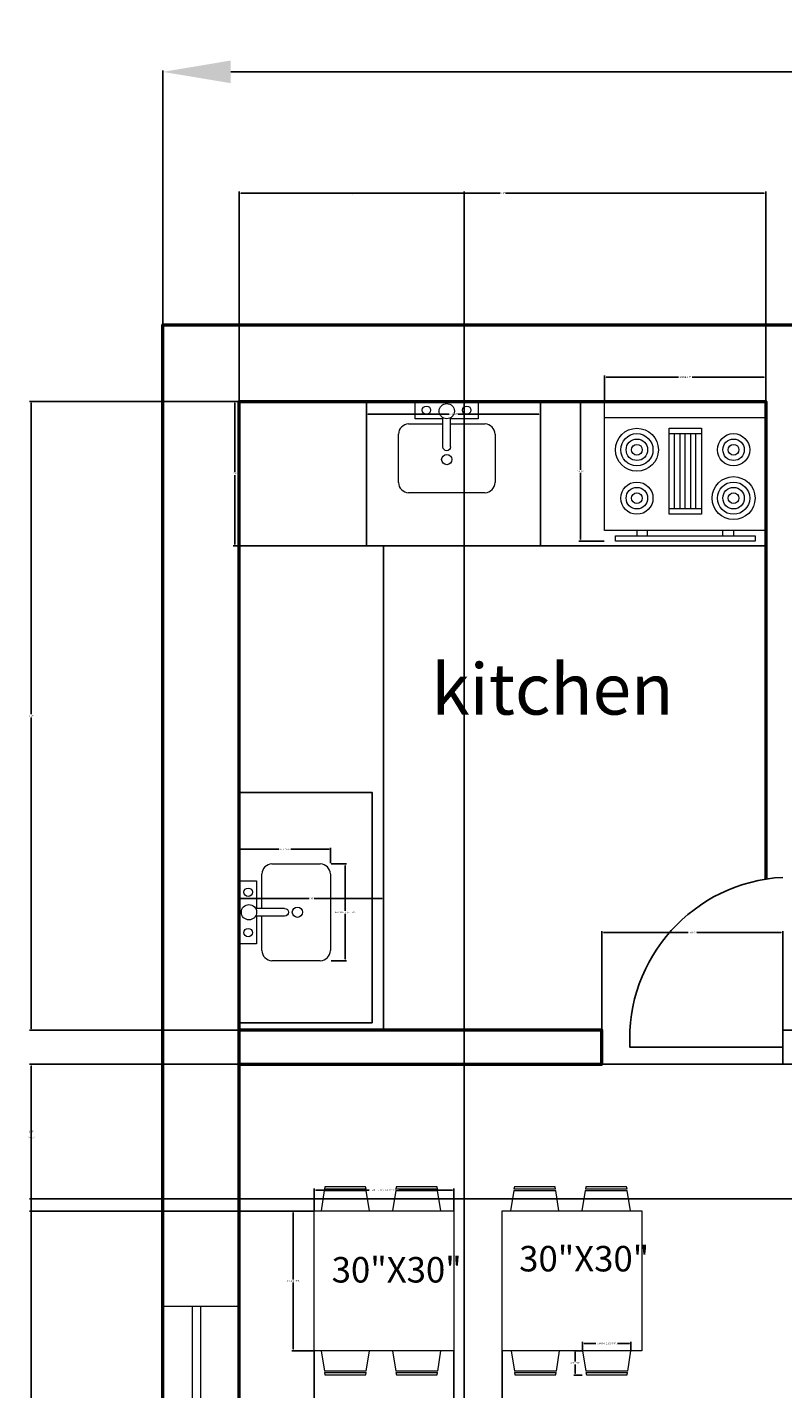
# Model space of a CAD drawing. Units: inches. Extents: x 226 to 1155, y 22 to 494.
# Tile 2 of 7: x 226 to 315, y 176 to 337. Entities that reach past the tile are written whole.
import ezdxf

# ---------------------------------------------------------------- set-up
doc = ezdxf.new("R2010")
doc.units = ezdxf.units.IN
doc.header["$MEASUREMENT"] = 0
for name, color, linetype, lineweight in [('A-ANNO-DIMS', 2, 'Continuous', 18), ('A-ANNO-TEXT', 7, 'Continuous', 18), ('A-AREA-IDEN', 7, 'Continuous', 25), ('A-DOOR', 3, 'Continuous', 25), ('A-EQPM', 8, 'Continuous', 18), ('A-FLOR-CASE', 9, 'Continuous', 25), ('A-FLOR-FIXT', 9, 'Continuous', 18), ('A-FURN', 8, 'Continuous', 18), ('A-GLAZ', 4, 'Continuous', 18), ('A-WALL', 7, 'Continuous', 50)]:
    doc.layers.add(name, color=color, linetype=linetype, lineweight=lineweight)
doc.styles.get("Standard").update_dxf_attribs({"font": 'arial.ttf'})
doc.dimstyles.get("Standard").update_dxf_attribs({"dimtxt": 0.18, "dimasz": 0.18, "dimexe": 0.18, "dimexo": 0.0625, "dimgap": 0.09, "dimtad": 0, "dimtih": 1, "dimtoh": 1, "dimdec": 4, "dimzin": 0, "dimdsep": 46, "dimlunit": 4, "dimtxsty": 'Standard', "dimcen": 0.09, "dimadec": 0, "dimazin": 0, "dimtfac": 1, "dimtdec": 4, "dimtofl": 0, "dimtmove": 0, "dimatfit": 3, "dimfxl": 1, "dimtolj": 1, "dimtzin": 0, "dimarcsym": 0})

# ---------------------------------------------------------------- blocks, each defined once
blk = doc.blocks.new('Range-Oven - 30 in top')
for p, q in [((0, -3), (30, -3)), ((12, -6), (18, -6)), ((13, -20), (13, -6)), ((14, -6), (14, -20)), ((15, -20), (15, -6)), ((16, -6), (16, -20)), ((17, -20), (17, -6)), ((18, -20), (12, -20)), ((6, -24), (6, -25)), ((8, -25), (8, -24)), ((22, -25), (22, -24)), ((24, -24), (24, -25))]:
    blk.add_line(p, q)
for points in [[(0, -24), (0, 0), (30, 0), (30, -24)], [(12, -21), (12, -5), (18, -5), (18, -21)], [(2, -26), (2, -25), (28, -25), (28, -26)]]:
    blk.add_lwpolyline(points, close=True)
for centre, radius in [((6, -9), 4), ((6, -9), 3), ((6, -9), 2), ((24, -9), 3), ((24, -9), 2), ((6, -9), 1), ((24, -9), 1), ((6, -18), 3), ((24, -18), 4), ((24, -18), 3), ((6, -18), 2), ((6, -18), 1), ((24, -18), 2), ((24, -18), 1)]:
    blk.add_circle(centre, radius)
blk = doc.blocks.new('*D9')
at = {"layer": 'A-ANNO-DIMS', "color": 0, "lineweight": -2, "transparency": 16777216}
for p, q in [((241.71, 301.69), (241.71, 331.58)), ((249.71, 331.4), (325.2, 331.4)), ((413.71, 331.4), (338.21, 331.4)), ((421.71, 301.69), (421.71, 331.58))]:
    blk.add_line(p, q, dxfattribs=at)
at = {"layer": 'A-ANNO-DIMS', "color": 0, "transparency": 16777216}
for points in [[(249.71, 332.74), (249.71, 330.07), (241.71, 331.4)], [(413.71, 332.74), (413.71, 330.07), (421.71, 331.4)]]:
    blk.add_solid(points, dxfattribs=at)
at = {"layer": 'Defpoints', "color": 0, "transparency": 16777216}
for p in [(421.71, 331.4), (241.71, 301.63), (421.71, 301.63)]:
    blk.add_point(p, dxfattribs=at)
at = {"layer": 'A-ANNO-DIMS', "color": 0, "transparency": 16777216, "insert": (331.71, 331.4), "char_height": 8, "attachment_point": 5}
blk.add_mtext("\\A1;15'", dxfattribs=at)
blk = doc.blocks.new('CHAIR-DINING-COMPACT')
for p, q in [((0.38, 2.4), (0, 0)), ((0.38, 2.4), (5.32, 2.4)), ((5.3, 2.55), (0.4, 2.55)), ((5.7, 0), (5.32, 2.4))]:
    blk.add_line(p, q)
blk.add_lwpolyline([(5.3, 2.55), (5.25, 2.85), (0.45, 2.85), (0.4, 2.55)])
blk = doc.blocks.new('TABLE-DINING-SQ-SMALL')
blk.add_lwpolyline([(0, 16.45), (16.45, 16.45), (16.45, 0), (0, 0)], close=True)
blk = doc.blocks.new('BASIN-WITH-FAUCET')
blk.add_line((6.15, 5.4), (6.15, 8.82))
for points in [[(5.25, 8.7), (2, 8.7), (2, 10.75), (5.8, 10.75)], [(5.8, 10.75), (9.4, 10.75), (9.4, 8.7), (6.15, 8.7)], [(1.2, 8.1), (5.25, 8.1)], [(6.15, 8.1), (10.2, 8.1)], [(0, 1.2), (0, 6.9)], [(11.4, 6.9), (11.4, 1.2)], [(10.2, 0), (1.2, 0)]]:
    blk.add_lwpolyline(points)
blk.add_lwpolyline([(6.15, 5.4, -1), (5.25, 5.4), (5.25, 8.82)], format="xyb")
for centre, radius in [((3.3, 9.7), 0.5), ((5.7, 9.6), 0.9), ((8.05, 9.7), 0.5), ((5.7, 3.9), 0.6)]:
    blk.add_circle(centre, radius)
for centre, start, end in [((1.28, 6.82), 93.3665, 176.6335), ((10.13, 6.82), 3.3665, 86.6335), ((1.28, 1.27), 183.3665, 266.6335), ((10.13, 1.27), 273.3665, 356.6335)]:
    blk.add_arc(centre, 1.28, start, end)
blk = doc.blocks.new('WIN-120-SLIDING')
blk.add_lwpolyline([(9, 0), (0, 0), (0, 120), (9, 120)], close=True)
for points in [[(5.5, 0), (5.5, 60), (4.5, 60), (3.5, 60), (3.5, 120)], [(4.5, 0), (4.5, 60), (4.5, 120)]]:
    blk.add_lwpolyline(points)
blk = doc.blocks.new('*D24')
at = {"layer": 'A-ANNO-DIMS', "color": 0, "lineweight": -2, "transparency": 16777216}
for p, q in [((291.14, 180.99), (291.14, 181.96)), ((291.32, 181.78), (292.71, 181.78)), ((296.65, 181.78), (295.26, 181.78)), ((296.83, 180.99), (296.83, 181.96))]:
    blk.add_line(p, q, dxfattribs=at)
at = {"layer": 'A-ANNO-DIMS', "color": 0, "transparency": 16777216}
for points in [[(291.32, 181.81), (291.32, 181.75), (291.14, 181.78)], [(296.65, 181.81), (296.65, 181.75), (296.83, 181.78)]]:
    blk.add_solid(points, dxfattribs=at)
at = {"layer": 'Defpoints', "color": 0, "transparency": 16777216}
for p in [(291.14, 181.78), (291.14, 180.93), (296.83, 180.93)]:
    blk.add_point(p, dxfattribs=at)
at = {"layer": 'A-ANNO-DIMS', "color": 0, "transparency": 16777216, "insert": (293.98, 181.78), "char_height": 0.18, "attachment_point": 5}
blk.add_mtext('\\A1;CHAIR 0\'-5 1/2" TYP.', dxfattribs=at)
blk = doc.blocks.new('*D25')
at = {"layer": 'A-ANNO-DIMS', "color": 0, "lineweight": -2, "transparency": 16777216}
for p, q in [((291.07, 180.93), (290.1, 180.93)), ((290.28, 180.75), (290.28, 179.68)), ((291.07, 178.07), (290.1, 178.07)), ((290.28, 178.25), (290.28, 179.32))]:
    blk.add_line(p, q, dxfattribs=at)
at = {"layer": 'A-ANNO-DIMS', "color": 0, "transparency": 16777216}
for points in [[(290.25, 180.75), (290.31, 180.75), (290.28, 180.93)], [(290.25, 178.25), (290.31, 178.25), (290.28, 178.07)]]:
    blk.add_solid(points, dxfattribs=at)
at = {"layer": 'Defpoints', "color": 0, "transparency": 16777216}
for p in [(291.14, 180.93), (290.28, 178.07), (291.14, 178.07)]:
    blk.add_point(p, dxfattribs=at)
at = {"layer": 'A-ANNO-DIMS', "color": 0, "transparency": 16777216, "insert": (290.28, 179.5), "char_height": 0.18, "attachment_point": 5}
blk.add_mtext('\\A1;0\'-3" TYP.', dxfattribs=at)
blk = doc.blocks.new('*D30')
at = {"layer": 'A-ANNO-DIMS', "color": 0, "lineweight": -2, "transparency": 16777216}
for p, q in [((261.52, 238.22), (263.35, 238.22)), ((263.17, 238.04), (263.17, 232.7)), ((263.17, 227), (263.17, 232.34)), ((261.52, 226.82), (263.35, 226.82))]:
    blk.add_line(p, q, dxfattribs=at)
at = {"layer": 'A-ANNO-DIMS', "color": 0, "transparency": 16777216}
for points in [[(263.14, 238.04), (263.2, 238.04), (263.17, 238.22)], [(263.14, 227), (263.2, 227), (263.17, 226.82)]]:
    blk.add_solid(points, dxfattribs=at)
at = {"layer": 'Defpoints', "color": 0, "transparency": 16777216}
for p in [(261.46, 238.22), (263.17, 238.22), (261.46, 226.82)]:
    blk.add_point(p, dxfattribs=at)
at = {"layer": 'A-ANNO-DIMS', "color": 0, "transparency": 16777216, "insert": (263.17, 232.52), "char_height": 0.18, "attachment_point": 5}
blk.add_mtext('\\A1;BASIN 0\'-11 1/2" TYP.', dxfattribs=at)
blk = doc.blocks.new('*D31')
at = {"layer": 'A-ANNO-DIMS', "color": 0, "lineweight": -2, "transparency": 16777216}
for p, q in [((250.71, 238.28), (250.71, 240.11)), ((250.89, 239.93), (255.37, 239.93)), ((261.28, 239.93), (256.79, 239.93)), ((261.46, 238.28), (261.46, 240.11))]:
    blk.add_line(p, q, dxfattribs=at)
at = {"layer": 'A-ANNO-DIMS', "color": 0, "transparency": 16777216}
for points in [[(250.89, 239.96), (250.89, 239.9), (250.71, 239.93)], [(261.28, 239.96), (261.28, 239.9), (261.46, 239.93)]]:
    blk.add_solid(points, dxfattribs=at)
at = {"layer": 'Defpoints', "color": 0, "transparency": 16777216}
for p in [(250.71, 239.93), (250.71, 238.22), (261.46, 238.22)]:
    blk.add_point(p, dxfattribs=at)
at = {"layer": 'A-ANNO-DIMS', "color": 0, "transparency": 16777216, "insert": (256.08, 239.93), "char_height": 0.18, "attachment_point": 5}
blk.add_mtext('\\A1;0\'-11" TYP.', dxfattribs=at)
blk = doc.blocks.new('*D38')
at = {"layer": 'A-ANNO-DIMS', "color": 0, "lineweight": -2, "transparency": 16777216}
for p, q in [((259.54, 197.44), (259.54, 200.02)), ((259.72, 199.84), (266.02, 199.84)), ((275.8, 199.84), (269.51, 199.84)), ((275.98, 197.44), (275.98, 200.02))]:
    blk.add_line(p, q, dxfattribs=at)
at = {"layer": 'A-ANNO-DIMS', "color": 0, "transparency": 16777216}
for points in [[(259.72, 199.87), (259.72, 199.81), (259.54, 199.84)], [(275.8, 199.87), (275.8, 199.81), (275.98, 199.84)]]:
    blk.add_solid(points, dxfattribs=at)
at = {"layer": 'Defpoints', "color": 0, "transparency": 16777216}
for p in [(275.98, 199.84), (259.54, 197.37), (275.98, 197.37)]:
    blk.add_point(p, dxfattribs=at)
at = {"layer": 'A-ANNO-DIMS', "color": 0, "transparency": 16777216, "insert": (267.76, 199.84), "char_height": 0.18, "attachment_point": 5}
blk.add_mtext('\\A1;TABLE BLOCK 1\'-4 1/2" TYP.', dxfattribs=at)
blk = doc.blocks.new('*D39')
at = {"layer": 'A-ANNO-DIMS', "color": 0, "lineweight": -2, "transparency": 16777216}
for p, q in [((259.47, 197.37), (256.89, 197.37)), ((257.07, 197.19), (257.07, 189.33)), ((257.07, 181.11), (257.07, 188.97)), ((259.47, 180.93), (256.89, 180.93))]:
    blk.add_line(p, q, dxfattribs=at)
at = {"layer": 'A-ANNO-DIMS', "color": 0, "transparency": 16777216}
for points in [[(257.04, 197.19), (257.1, 197.19), (257.07, 197.37)], [(257.04, 181.11), (257.1, 181.11), (257.07, 180.93)]]:
    blk.add_solid(points, dxfattribs=at)
at = {"layer": 'Defpoints', "color": 0, "transparency": 16777216}
for p in [(257.07, 197.37), (259.54, 197.37), (259.54, 180.93)]:
    blk.add_point(p, dxfattribs=at)
at = {"layer": 'A-ANNO-DIMS', "color": 0, "transparency": 16777216, "insert": (257.07, 189.15), "char_height": 0.18, "attachment_point": 5}
blk.add_mtext('\\A1;1\'-4 1/2" TYP.', dxfattribs=at)
blk = doc.blocks.new('*D48')
at = {"layer": 'A-ANNO-DIMS', "color": 0, "lineweight": -2, "transparency": 16777216}
for p, q in [((293.73, 292.69), (293.73, 295.66)), ((293.91, 295.48), (302.41, 295.48)), ((312.53, 295.48), (304.03, 295.48)), ((312.71, 292.69), (312.71, 295.66))]:
    blk.add_line(p, q, dxfattribs=at)
at = {"layer": 'A-ANNO-DIMS', "color": 0, "transparency": 16777216}
for points in [[(293.91, 295.51), (293.91, 295.45), (293.73, 295.48)], [(312.53, 295.51), (312.53, 295.45), (312.71, 295.48)]]:
    blk.add_solid(points, dxfattribs=at)
at = {"layer": 'Defpoints', "color": 0, "transparency": 16777216}
for p in [(312.71, 295.48), (293.73, 292.63), (312.71, 292.63)]:
    blk.add_point(p, dxfattribs=at)
at = {"layer": 'A-ANNO-DIMS', "color": 0, "transparency": 16777216, "insert": (303.22, 295.48), "char_height": 0.18, "attachment_point": 5}
blk.add_mtext('\\A1;RANGE 1\'-7"', dxfattribs=at)
blk = doc.blocks.new('*D49')
at = {"layer": 'A-ANNO-DIMS', "color": 0, "lineweight": -2, "transparency": 16777216}
for p, q in [((293.67, 292.63), (290.71, 292.63)), ((290.89, 292.45), (290.89, 284.59)), ((290.89, 276.37), (290.89, 284.22)), ((293.67, 276.19), (290.71, 276.19))]:
    blk.add_line(p, q, dxfattribs=at)
at = {"layer": 'A-ANNO-DIMS', "color": 0, "transparency": 16777216}
for points in [[(290.86, 292.45), (290.92, 292.45), (290.89, 292.63)], [(290.86, 276.37), (290.92, 276.37), (290.89, 276.19)]]:
    blk.add_solid(points, dxfattribs=at)
at = {"layer": 'Defpoints', "color": 0, "transparency": 16777216}
for p in [(290.89, 292.63), (293.73, 292.63), (293.73, 276.19)]:
    blk.add_point(p, dxfattribs=at)
at = {"layer": 'A-ANNO-DIMS', "color": 0, "transparency": 16777216, "insert": (290.89, 284.41), "char_height": 0.18, "attachment_point": 5}
blk.add_mtext('\\A1;1\'-4 1/2"', dxfattribs=at)
blk = doc.blocks.new('*D56')
at = {"layer": 'A-ANNO-DIMS', "color": 0, "lineweight": -2, "transparency": 16777216}
for p, q in [((250.71, 292.69), (250.71, 317.31)), ((312.71, 292.69), (312.71, 317.31)), ((250.89, 317.13), (281.38, 317.13)), ((312.53, 317.13), (282.04, 317.13))]:
    blk.add_line(p, q, dxfattribs=at)
at = {"layer": 'A-ANNO-DIMS', "color": 0, "transparency": 16777216}
for points in [[(250.89, 317.16), (250.89, 317.1), (250.71, 317.13)], [(312.53, 317.16), (312.53, 317.1), (312.71, 317.13)]]:
    blk.add_solid(points, dxfattribs=at)
at = {"layer": 'Defpoints', "color": 0, "transparency": 16777216}
for p in [(312.71, 317.13), (250.71, 292.63), (312.71, 292.63)]:
    blk.add_point(p, dxfattribs=at)
at = {"layer": 'A-ANNO-DIMS', "color": 0, "transparency": 16777216, "insert": (281.71, 317.13), "char_height": 0.18, "attachment_point": 5}
blk.add_mtext('\\A1;5\'-2"', dxfattribs=at)
blk = doc.blocks.new('*D59')
at = {"layer": 'A-ANNO-DIMS', "color": 0, "lineweight": -2, "transparency": 16777216}
for p, q in [((250.64, 292.63), (226.03, 292.63)), ((226.21, 292.45), (226.21, 255.81)), ((226.21, 218.81), (226.21, 255.45)), ((250.64, 218.63), (226.03, 218.63))]:
    blk.add_line(p, q, dxfattribs=at)
at = {"layer": 'A-ANNO-DIMS', "color": 0, "transparency": 16777216}
for points in [[(226.18, 292.45), (226.24, 292.45), (226.21, 292.63)], [(226.18, 218.81), (226.24, 218.81), (226.21, 218.63)]]:
    blk.add_solid(points, dxfattribs=at)
at = {"layer": 'Defpoints', "color": 0, "transparency": 16777216}
for p in [(250.71, 292.63), (226.21, 218.63), (250.71, 218.63)]:
    blk.add_point(p, dxfattribs=at)
at = {"layer": 'A-ANNO-DIMS', "color": 0, "transparency": 16777216, "insert": (226.21, 255.63), "char_height": 0.18, "attachment_point": 5}
blk.add_mtext('\\A1;6\'-2"', dxfattribs=at)
blk = doc.blocks.new('*D67')
at = {"layer": 'A-ANNO-DIMS', "color": 0, "lineweight": -2, "transparency": 16777216}
for p, q in [((250.64, 214.63), (226.03, 214.63)), ((226.21, 214.45), (226.21, 130.81)), ((226.21, 46.81), (226.21, 130.45)), ((250.64, 46.63), (226.03, 46.63))]:
    blk.add_line(p, q, dxfattribs=at)
at = {"layer": 'A-ANNO-DIMS', "color": 0, "transparency": 16777216}
for points in [[(226.18, 214.45), (226.24, 214.45), (226.21, 214.63)], [(226.18, 46.81), (226.24, 46.81), (226.21, 46.63)]]:
    blk.add_solid(points, dxfattribs=at)
at = {"layer": 'Defpoints', "color": 0, "transparency": 16777216}
for p in [(226.21, 214.63), (250.71, 214.63), (250.71, 46.63)]:
    blk.add_point(p, dxfattribs=at)
at = {"layer": 'A-ANNO-DIMS', "color": 0, "transparency": 16777216, "insert": (226.21, 130.63), "char_height": 0.18, "attachment_point": 5}
blk.add_mtext('\\A1;14\'-0"', dxfattribs=at)
blk = doc.blocks.new('*D69')
at = {"layer": 'A-ANNO-DIMS', "color": 0, "lineweight": -2, "transparency": 16777216}
for p, q in [((250.71, 46.69), (250.71, 317.31)), ((277.18, 80.75), (277.18, 317.31)), ((250.89, 317.13), (263.4, 317.13)), ((277, 317.13), (264.48, 317.13))]:
    blk.add_line(p, q, dxfattribs=at)
at = {"layer": 'A-ANNO-DIMS', "color": 0, "transparency": 16777216}
for points in [[(250.89, 317.16), (250.89, 317.1), (250.71, 317.13)], [(277, 317.16), (277, 317.1), (277.18, 317.13)]]:
    blk.add_solid(points, dxfattribs=at)
at = {"layer": 'Defpoints', "color": 0, "transparency": 16777216}
for p in [(277.18, 317.13), (277.18, 80.69), (250.71, 46.63)]:
    blk.add_point(p, dxfattribs=at)
at = {"layer": 'A-ANNO-DIMS', "color": 0, "transparency": 16777216, "insert": (263.94, 317.13), "char_height": 0.18, "attachment_point": 5}
blk.add_mtext('\\A1;2\'-2 1/2"', dxfattribs=at)
blk = doc.blocks.new('*D71')
at = {"layer": 'A-ANNO-DIMS', "color": 0, "lineweight": -2, "transparency": 16777216}
for p, q in [((241.71, 301.57), (241.71, 21.95)), ((322.71, 301.57), (322.71, 21.95)), ((241.89, 22.13), (281.88, 22.13)), ((322.53, 22.13), (282.54, 22.13))]:
    blk.add_line(p, q, dxfattribs=at)
at = {"layer": 'A-ANNO-DIMS', "color": 0, "transparency": 16777216}
for points in [[(241.89, 22.16), (241.89, 22.1), (241.71, 22.13)], [(322.53, 22.16), (322.53, 22.1), (322.71, 22.13)]]:
    blk.add_solid(points, dxfattribs=at)
at = {"layer": 'Defpoints', "color": 0, "transparency": 16777216}
for p in [(241.71, 301.63), (322.71, 301.63), (322.71, 22.13)]:
    blk.add_point(p, dxfattribs=at)
at = {"layer": 'A-ANNO-DIMS', "color": 0, "transparency": 16777216, "insert": (282.21, 22.13), "char_height": 0.18, "attachment_point": 5}
blk.add_mtext('\\A1;6\'-9"', dxfattribs=at)
blk = doc.blocks.new('*D78')
at = {"layer": 'A-ANNO-DIMS', "color": 0, "lineweight": -2, "transparency": 16777216}
for p, q in [((250.64, 214.63), (226.03, 214.63)), ((226.21, 214.45), (226.21, 206.19)), ((226.21, 197.55), (226.21, 205.82)), ((259.47, 197.37), (226.03, 197.37))]:
    blk.add_line(p, q, dxfattribs=at)
at = {"layer": 'A-ANNO-DIMS', "color": 0, "transparency": 16777216}
for points in [[(226.18, 214.45), (226.24, 214.45), (226.21, 214.63)], [(226.18, 197.55), (226.24, 197.55), (226.21, 197.37)]]:
    blk.add_solid(points, dxfattribs=at)
at = {"layer": 'Defpoints', "color": 0, "transparency": 16777216}
for p in [(250.71, 214.63), (226.21, 197.37), (259.54, 197.37)]:
    blk.add_point(p, dxfattribs=at)
at = {"layer": 'A-ANNO-DIMS', "color": 0, "transparency": 16777216, "insert": (226.21, 206), "char_height": 0.18, "attachment_point": 5}
blk.add_mtext('\\A1;1\'-5 1/2"', dxfattribs=at)
blk = doc.blocks.new('*D79')
at = {"layer": 'A-ANNO-DIMS', "color": 0, "lineweight": -2, "transparency": 16777216}
for p, q in [((250.71, 186.1), (250.71, 21.95)), ((259.54, 180.86), (259.54, 21.95)), ((250.89, 22.13), (254.79, 22.13)), ((259.36, 22.13), (255.45, 22.13))]:
    blk.add_line(p, q, dxfattribs=at)
at = {"layer": 'A-ANNO-DIMS', "color": 0, "transparency": 16777216}
for points in [[(250.89, 22.16), (250.89, 22.1), (250.71, 22.13)], [(259.36, 22.16), (259.36, 22.1), (259.54, 22.13)]]:
    blk.add_solid(points, dxfattribs=at)
at = {"layer": 'Defpoints', "color": 0, "transparency": 16777216}
for p in [(250.71, 186.17), (259.54, 180.93), (259.54, 22.13)]:
    blk.add_point(p, dxfattribs=at)
at = {"layer": 'A-ANNO-DIMS', "color": 0, "transparency": 16777216, "insert": (255.12, 22.13), "char_height": 0.18, "attachment_point": 5}
blk.add_mtext('\\A1;0\'-9"', dxfattribs=at)
blk = doc.blocks.new('*D80')
at = {"layer": 'A-ANNO-DIMS', "color": 0, "lineweight": -2, "transparency": 16777216}
for p, q in [((275.98, 180.86), (275.98, 21.95)), ((281.68, 180.86), (281.68, 21.95)), ((276.16, 22.13), (278.29, 22.13)), ((281.5, 22.13), (279.37, 22.13))]:
    blk.add_line(p, q, dxfattribs=at)
at = {"layer": 'A-ANNO-DIMS', "color": 0, "transparency": 16777216}
for points in [[(276.16, 22.16), (276.16, 22.1), (275.98, 22.13)], [(281.5, 22.16), (281.5, 22.1), (281.68, 22.13)]]:
    blk.add_solid(points, dxfattribs=at)
at = {"layer": 'Defpoints', "color": 0, "transparency": 16777216}
for p in [(275.98, 180.93), (281.68, 180.93), (281.68, 22.13)]:
    blk.add_point(p, dxfattribs=at)
at = {"layer": 'A-ANNO-DIMS', "color": 0, "transparency": 16777216, "insert": (278.83, 22.13), "char_height": 0.18, "attachment_point": 5}
blk.add_mtext('\\A1;0\'-5 1/2"', dxfattribs=at)
blk = doc.blocks.new('*D82')
at = {"layer": 'A-ANNO-DIMS', "color": 0, "lineweight": -2, "transparency": 16777216}
for p, q in [((357.96, 214.63), (226.03, 214.63)), ((226.21, 214.45), (226.21, 206.9)), ((226.21, 199), (226.21, 206.54)), ((357.96, 198.82), (226.03, 198.82))]:
    blk.add_line(p, q, dxfattribs=at)
at = {"layer": 'A-ANNO-DIMS', "color": 0, "transparency": 16777216}
for points in [[(226.18, 214.45), (226.24, 214.45), (226.21, 214.63)], [(226.18, 199), (226.24, 199), (226.21, 198.82)]]:
    blk.add_solid(points, dxfattribs=at)
at = {"layer": 'Defpoints', "color": 0, "transparency": 16777216}
for p in [(226.21, 214.63), (358.02, 214.63), (358.02, 198.82)]:
    blk.add_point(p, dxfattribs=at)
at = {"layer": 'A-ANNO-DIMS', "color": 0, "transparency": 16777216, "insert": (226.21, 206.72), "char_height": 0.18, "attachment_point": 5}
blk.add_mtext('\\A1;1\'-4"', dxfattribs=at)
blk = doc.blocks.new('*D86')
at = {"layer": 'A-ANNO-DIMS', "color": 0, "lineweight": -2, "transparency": 16777216}
for p, q in [((250.71, 218.69), (250.71, 234.31)), ((250.89, 234.13), (258.89, 234.13)), ((267.53, 234.13), (259.53, 234.13)), ((267.71, 218.69), (267.71, 234.31))]:
    blk.add_line(p, q, dxfattribs=at)
at = {"layer": 'A-ANNO-DIMS', "color": 0, "transparency": 16777216}
for points in [[(250.89, 234.16), (250.89, 234.1), (250.71, 234.13)], [(267.53, 234.16), (267.53, 234.1), (267.71, 234.13)]]:
    blk.add_solid(points, dxfattribs=at)
at = {"layer": 'Defpoints', "color": 0, "transparency": 16777216}
for p in [(267.71, 234.13), (250.71, 218.63), (267.71, 218.63)]:
    blk.add_point(p, dxfattribs=at)
at = {"layer": 'A-ANNO-DIMS', "color": 0, "transparency": 16777216, "insert": (259.21, 234.13), "char_height": 0.18, "attachment_point": 5}
blk.add_mtext('\\A1;1\'-5"', dxfattribs=at)
blk = doc.blocks.new('*D87')
at = {"layer": 'A-ANNO-DIMS', "color": 0, "lineweight": -2, "transparency": 16777216}
for p, q in [((265.62, 292.63), (250, 292.63)), ((250.18, 292.45), (250.18, 284.31)), ((250.18, 275.81), (250.18, 283.95)), ((265.62, 275.63), (250, 275.63))]:
    blk.add_line(p, q, dxfattribs=at)
at = {"layer": 'A-ANNO-DIMS', "color": 0, "transparency": 16777216}
for points in [[(250.15, 292.45), (250.21, 292.45), (250.18, 292.63)], [(250.15, 275.81), (250.21, 275.81), (250.18, 275.63)]]:
    blk.add_solid(points, dxfattribs=at)
at = {"layer": 'Defpoints', "color": 0, "transparency": 16777216}
for p in [(250.18, 292.63), (265.68, 292.63), (265.68, 275.63)]:
    blk.add_point(p, dxfattribs=at)
at = {"layer": 'A-ANNO-DIMS', "color": 0, "transparency": 16777216, "insert": (250.18, 284.13), "char_height": 0.18, "attachment_point": 5}
blk.add_mtext('\\A1;1\'-5"', dxfattribs=at)
blk = doc.blocks.new('*D88')
at = {"layer": 'A-ANNO-DIMS', "color": 0, "lineweight": -2, "transparency": 16777216}
for p, q in [((265.68, 275.69), (265.68, 291.31)), ((265.86, 291.13), (275.39, 291.13)), ((285.99, 291.13), (276.45, 291.13)), ((286.17, 275.69), (286.17, 291.31))]:
    blk.add_line(p, q, dxfattribs=at)
at = {"layer": 'A-ANNO-DIMS', "color": 0, "transparency": 16777216}
for points in [[(265.86, 291.16), (265.86, 291.1), (265.68, 291.13)], [(285.99, 291.16), (285.99, 291.1), (286.17, 291.13)]]:
    blk.add_solid(points, dxfattribs=at)
at = {"layer": 'Defpoints', "color": 0, "transparency": 16777216}
for p in [(286.17, 291.13), (265.68, 275.63), (286.17, 275.63)]:
    blk.add_point(p, dxfattribs=at)
at = {"layer": 'A-ANNO-DIMS', "color": 0, "transparency": 16777216, "insert": (275.92, 291.13), "char_height": 0.18, "attachment_point": 5}
blk.add_mtext('\\A1;1\'-8 1/2"', dxfattribs=at)
blk = doc.blocks.new('*D89')
at = {"layer": 'A-ANNO-DIMS', "color": 0, "lineweight": -2, "transparency": 16777216}
for p, q in [((293.4, 214.69), (293.4, 230.31)), ((293.58, 230.13), (303.52, 230.13)), ((314.53, 230.13), (304.58, 230.13)), ((314.71, 214.69), (314.71, 230.31))]:
    blk.add_line(p, q, dxfattribs=at)
at = {"layer": 'A-ANNO-DIMS', "color": 0, "transparency": 16777216}
for points in [[(293.58, 230.16), (293.58, 230.1), (293.4, 230.13)], [(314.53, 230.16), (314.53, 230.1), (314.71, 230.13)]]:
    blk.add_solid(points, dxfattribs=at)
at = {"layer": 'Defpoints', "color": 0, "transparency": 16777216}
for p in [(314.71, 230.13), (293.4, 214.63), (314.71, 214.63)]:
    blk.add_point(p, dxfattribs=at)
at = {"layer": 'A-ANNO-DIMS', "color": 0, "transparency": 16777216, "insert": (304.05, 230.13), "char_height": 0.18, "attachment_point": 5}
blk.add_mtext('\\A1;1\'-9 1/2"', dxfattribs=at)

msp = doc.modelspace()

# ---------------------------------------------------------------- linework, layer by layer
at = {"layer": 'A-DOOR'}
msp.add_lwpolyline([(314.70585, 236.62988, 0.414213562), (296.70585, 216.62988), (296.70585, 218.62988)], format="xyb", dxfattribs=at)
msp.add_lwpolyline([(320.70585, 218.62988), (314.70585, 218.62988), (314.70585, 216.62988), (296.70585, 216.62988)], dxfattribs=at)
at = {"layer": 'A-FLOR-CASE'}
for points in [[(265.67802, 292.62988), (286.16593, 292.62988), (286.16593, 275.62988), (265.67802, 275.62988)], [(250.70585, 246.62988), (266.35613, 246.62988), (266.35613, 219.52279), (250.70585, 219.52279)]]:
    msp.add_lwpolyline(points, close=True, dxfattribs=at)
msp.add_lwpolyline([(312.70585, 275.62988), (267.70585, 275.62988), (267.70585, 218.62988)], dxfattribs=at)
at = {"layer": 'A-WALL'}
for points in [[(307.38052, 37.62988), (241.70585, 37.62988), (241.70585, 301.62988), (421.70585, 301.62988), (421.70585, 37.62988), (351.38052, 37.62988)], [(309.38052, 46.62988), (250.70585, 46.62988), (250.70585, 292.62988), (312.70585, 292.62988), (312.70585, 236.41817)], [(250.70585, 214.62988), (293.40183, 214.62988), (293.40183, 218.62988), (250.70585, 218.62988)]]:
    msp.add_lwpolyline(points, dxfattribs=at)

# ---------------------------------------------------------------- block references
at = {"layer": 'A-EQPM', "xscale": 0.6324555446827858, "yscale": 0.6324555446827858, "zscale": 0.6324555446827858}
msp.add_blockref('Range-Oven - 30 in top', (293.73218, 292.62988), dxfattribs=at)
at = {"layer": 'A-FLOR-FIXT'}
msp.add_blockref('BASIN-WITH-FAUCET', (269.44114, 281.88), dxfattribs=at)
at = {"layer": 'A-FLOR-FIXT', "rotation": 89.99999999999964}
msp.add_blockref('BASIN-WITH-FAUCET', (261.45572, 226.82159), dxfattribs=at)
at = {"layer": 'A-FURN'}
for name, p in [('CHAIR-DINING-COMPACT', (260.34123, 197.375)), ('CHAIR-DINING-COMPACT', (268.748, 197.375)), ('CHAIR-DINING-COMPACT', (282.65695, 197.375)), ('CHAIR-DINING-COMPACT', (291.06372, 197.375)), ('TABLE-DINING-SQ-SMALL', (259.536, 180.926)), ('TABLE-DINING-SQ-SMALL', (281.67681, 180.926))]:
    msp.add_blockref(name, p, dxfattribs=at)
at = {"layer": 'A-FURN', "rotation": 180}
for p in [(266.04806, 180.92579), (274.45483, 180.92579), (288.42444, 180.92579), (296.83121, 180.92579)]:
    msp.add_blockref('CHAIR-DINING-COMPACT', p, dxfattribs=at)
at = {"layer": 'A-GLAZ'}
msp.add_blockref('WIN-120-SLIDING', (241.706, 66.167), dxfattribs=at)

# ---------------------------------------------------------------- texts
at = {"layer": 'A-ANNO-TEXT', "char_height": 3, "attachment_point": 1}
for s, width, insert in [('30"X30"', 11.6185971, (283.66681, 193.26195)), ('30"X30"\\P ', 14.3931298, (261.59148, 191.95593))]:
    msp.add_mtext_dynamic_manual_height_columns(s, width=width, gutter_width=1, heights=[0], dxfattribs=dict(at, insert=insert))
at = {"layer": 'A-AREA-IDEN', "insert": (273.31311, 261.77848), "char_height": 6, "attachment_point": 1}
msp.add_mtext_dynamic_manual_height_columns('kitchen', width=39.3927311, gutter_width=1, heights=[0], dxfattribs=at)

# ---------------------------------------------------------------- dimensions: what is measured, and where the dimension line sits
at = {"layer": 'A-ANNO-DIMS'}
for base, p1, p2, override, picture, middle in [((421.70585, 331.40497), (241.70585, 301.62988), (421.70585, 301.62988), {"dimtxt": 8, "dimasz": 8, "dimclrd": 0, "dimclre": 0, "dimclrt": 0}, '*D9', (331.70585, 331.40497)), ((277.18287, 317.12988), (250.70585, 46.62988), (277.18287, 80.68669), {"dimdec": 1, "dimlfac": 1, "dimrnd": 0, "dimzin": 1, "dimdsep": 46, "dimlunit": 4, "dimfrac": 2}, '*D69', (263.94436, 317.12988)), ((312.70585, 317.12988), (250.70585, 292.62988), (312.70585, 292.62988), {"dimdec": 1, "dimlfac": 1, "dimrnd": 0, "dimzin": 1, "dimdsep": 46, "dimlunit": 4, "dimfrac": 2}, '*D56', (281.70585, 317.12988)), ((322.7094, 22.12988), (241.70585, 301.62988), (322.7094, 301.62988), {"dimdec": 1, "dimlfac": 1, "dimrnd": 0, "dimzin": 1, "dimdsep": 46, "dimlunit": 4, "dimfrac": 2}, '*D71', (282.20762, 22.12988)), ((286.16593, 291.12988), (265.67802, 275.62988), (286.16593, 275.62988), {"dimdec": 1, "dimlfac": 1, "dimrnd": 0, "dimzin": 1, "dimdsep": 46, "dimlunit": 4, "dimfrac": 2}, '*D88', (275.92197, 291.12988)), ((267.70585, 234.12988), (250.70585, 218.62988), (267.70585, 218.62988), {"dimdec": 1, "dimlfac": 1, "dimrnd": 0, "dimzin": 1, "dimdsep": 46, "dimlunit": 4, "dimfrac": 2}, '*D86', (259.20585, 234.12988)), ((259.53617, 22.12988), (250.70585, 186.1667), (259.53617, 180.92618), {"dimdec": 1, "dimlfac": 1, "dimrnd": 0, "dimzin": 1, "dimdsep": 46, "dimlunit": 4, "dimfrac": 2}, '*D79', (255.12101, 22.12988)), ((281.67698, 22.12988), (275.98461, 180.92618), (281.67698, 180.92618), {"dimdec": 1, "dimlfac": 1, "dimrnd": 0, "dimzin": 1, "dimdsep": 46, "dimlunit": 4, "dimfrac": 2}, '*D80', (278.8308, 22.12988))]:
    dim = msp.add_linear_dim(base=base, p1=p1, p2=p2, dimstyle='Standard', override=override, dxfattribs=at)
    dim.commit()
    dim.dimension.update_dxf_attribs({"geometry": picture, "text_midpoint": middle})
for base, p1, p2, text, picture, middle in [((312.70585, 295.47593), (293.73218, 292.62988), (312.70585, 292.62988), 'RANGE <>', '*D48', (303.21901, 295.47593)), ((275.98461, 199.84188), (259.53617, 197.37462), (275.98461, 197.37462), 'TABLE BLOCK <> TYP.', '*D38', (267.76039, 199.84188))]:
    dim = msp.add_linear_dim(base=base, p1=p1, p2=p2, text=text, dimstyle='Standard', override={"dimdec": 1, "dimlfac": 1, "dimrnd": 0, "dimzin": 1, "dimdsep": 46, "dimlunit": 4, "dimfrac": 2}, dxfattribs=at)
    dim.commit()
    dim.dimension.update_dxf_attribs({"geometry": picture, "text_midpoint": middle})
for base, p1, p2, angle, picture, middle in [((226.20585, 218.62988), (250.70585, 292.62988), (250.70585, 218.62988), 90, '*D59', (226.20585, 255.62988)), ((250.17802, 292.62988), (265.67802, 275.62988), (265.67802, 292.62988), 90, '*D87', (250.17802, 284.12988)), ((290.88613, 292.62988), (293.73218, 276.18604), (293.73218, 292.62988), 90, '*D49', (290.88613, 284.40796)), ((314.70585, 230.12988), (293.40183, 214.62988), (314.70585, 214.62988), 0, '*D89', (304.05384, 230.12988)), ((226.20585, 197.37462), (250.70585, 214.62988), (259.53617, 197.37462), 90, '*D78', (226.20585, 206.00225)), ((226.20585, 214.62988), (250.70585, 46.62988), (250.70585, 214.62988), 90, '*D67', (226.20585, 130.62988)), ((226.20585, 214.62988), (358.02219, 198.81719), (358.02219, 214.62988), 90, '*D82', (226.20585, 206.72354))]:
    dim = msp.add_linear_dim(base=base, p1=p1, p2=p2, angle=angle, dimstyle='Standard', override={"dimdec": 1, "dimlfac": 1, "dimrnd": 0, "dimzin": 1, "dimdsep": 46, "dimlunit": 4, "dimfrac": 2}, dxfattribs=at)
    dim.commit()
    dim.dimension.update_dxf_attribs({"geometry": picture, "text_midpoint": middle})
for base, p1, p2, angle, text, picture, middle in [((250.7058454797, 239.9319809144), (261.4558454797, 238.2219659144), (250.7058454797, 238.2219659144), 180, '<> TYP.', '*D31', (256.0808454797, 239.9319809144)), ((263.16586, 238.22197), (261.45585, 226.82187), (261.45585, 238.22197), 90, 'BASIN <> TYP.', '*D30', (263.16586, 232.52192)), ((257.0689, 197.37462), (259.53617, 180.92618), (259.53617, 197.37462), 90, '<> TYP.', '*D39', (257.0689, 189.1504)), ((291.13588, 181.78049), (296.83132, 180.92618), (291.13588, 180.92618), 180, 'CHAIR <> TYP.', '*D24', (293.9836, 181.78049)), ((290.28156, 178.07317), (291.13588, 180.92618), (291.13588, 178.07317), 270, '<> TYP.', '*D25', (290.28156, 179.49967))]:
    dim = msp.add_linear_dim(base=base, p1=p1, p2=p2, angle=angle, text=text, dimstyle='Standard', override={"dimdec": 1, "dimlfac": 1, "dimrnd": 0, "dimzin": 1, "dimdsep": 46, "dimlunit": 4, "dimfrac": 2}, dxfattribs=at)
    dim.commit()
    dim.dimension.update_dxf_attribs({"geometry": picture, "text_midpoint": middle})

doc.saveas('drawing.dxf')
